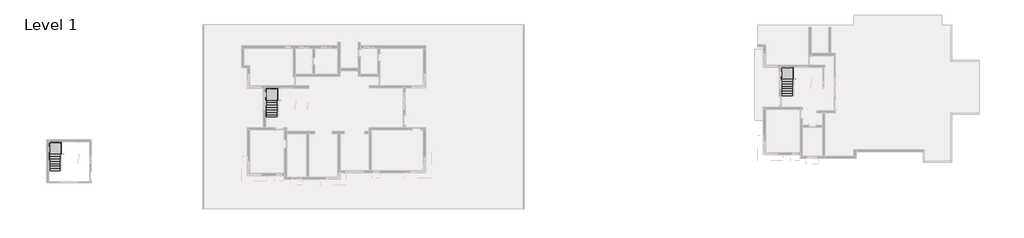
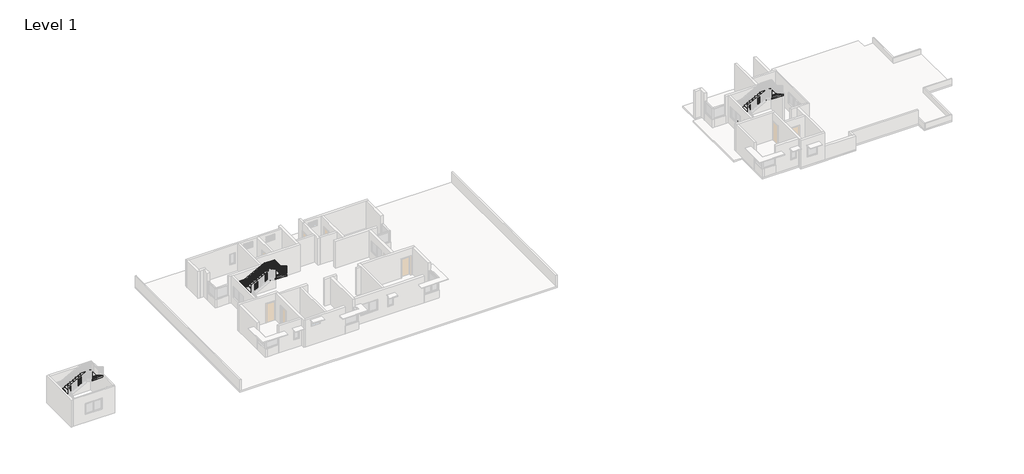
# One storey, part 7 of 9: 3 stair flights, 1 railing.
"""IFC4 building model written with IfcOpenShell, lengths in millimetres."""

from ifc_helpers import new_model, si_unit, frame, origin, place, context, project, spatial, polyline, outline, extrude, faceted_brep, transform, mapped, element, save
from components import stair_flight_18be0a75, stair_flight_c0b809fc, stair_flight_2ad91a83

model = new_model("IFC4")

# Units and contexts
model_context = context("Model", 3, world=origin())
ifc_project = project(units=[si_unit("LENGTHUNIT", "METRE", prefix="MILLI")], contexts=[model_context])

# Site, building, storey
site = spatial("IfcSite", under=ifc_project)
building = spatial("IfcBuilding", under=site)
storey = spatial("IfcBuildingStorey", under=building, Name="Level 1", Elevation=0.0)

# Railing
placement = place(None, origin())
element("IfcRailing", 1, ObjectType="Handrail - Rectangular", at=placement, inside=storey, context=model_context, shape_type="SolidModel", body=[
    faceted_brep([(-40950.9146233, 12415.3624892, 1059.5428571), (-40950.9146233, 12415.3624892, 1001.0339009), (-40900.1146233, 12415.3624892, 1001.0339009), (-40900.1146233, 12415.3624892, 1059.5428571), (-40950.9146233, 14360.1558226, 2170.8533333), (-40950.9146233, 14373.646496, 2120.0533333), (-40900.1146233, 14373.646496, 2120.0533333), (-40900.1146233, 14360.1558226, 2170.8533333), (-40950.9146233, 15412.5624892, 2170.8533333), (-40950.9146233, 15412.5624892, 2120.0533333), (-40900.1146233, 15361.7624892, 2120.0533333), (-40900.1146233, 15361.7624892, 2170.8533333), (-39825.1503376, 15412.5624892, 2170.8533333), (-39812.4503376, 15412.5624892, 2120.0533333), (-39812.4503376, 15361.7624892, 2120.0533333), (-39825.1503376, 15361.7624892, 2170.8533333), (-37733.2789091, 15412.5624892, 3286.5180952), (-37720.5789091, 15412.5624892, 3235.7180952), (-37720.5789091, 15361.7624892, 3235.7180952), (-37733.2789091, 15361.7624892, 3286.5180952), (-36607.5146233, 15412.5624892, 3286.5180952), (-36607.5146233, 15412.5624892, 3235.7180952), (-36658.3146233, 15361.7624892, 3235.7180952), (-36658.3146233, 15361.7624892, 3286.5180952), (-36607.5146233, 14360.1558226, 3286.5180952), (-36607.5146233, 14346.6651492, 3235.7180952), (-36658.3146233, 14346.6651492, 3235.7180952), (-36658.3146233, 14360.1558226, 3286.5180952), (-36607.5146233, 13177.3624892, 3962.4), (-36658.3146233, 13177.3624892, 3962.4), (-36658.3146233, 13177.3624892, 3903.8910438), (-36607.5146233, 13177.3624892, 3903.8910438)], [[[0, 1, 2, 3]], [[1, 0, 4, 5]], [[2, 1, 5, 6]], [[3, 2, 6, 7]], [[0, 3, 7, 4]], [[5, 4, 8, 9]], [[6, 5, 9, 10]], [[7, 6, 10, 11]], [[4, 7, 11, 8]], [[9, 8, 12, 13]], [[10, 9, 13, 14]], [[11, 10, 14, 15]], [[8, 11, 15, 12]], [[13, 12, 16, 17]], [[14, 13, 17, 18]], [[15, 14, 18, 19]], [[12, 15, 19, 16]], [[17, 16, 20, 21]], [[18, 17, 21, 22]], [[19, 18, 22, 23]], [[16, 19, 23, 20]], [[21, 20, 24, 25]], [[22, 21, 25, 26]], [[23, 22, 26, 27]], [[20, 23, 27, 24]], [[28, 29, 30, 31]], [[25, 24, 28, 31]], [[26, 25, 31, 30]], [[27, 26, 30, 29]], [[24, 27, 29, 28]]]),
    extrude(outline(polyline([(13263.0874892, 3854.9053295), (13263.0874892, 2902.8571429), (13244.0374892, 2902.8571429), (13244.0374892, 3865.7910438), (13263.0874892, 3854.9053295)])), frame((-36642.4396233, 0.0, 0.0), z_axis=(1.0, 0.0, 0.0), x_axis=(0.0, 1.0, 0.0)), (0.0, 0.0, 1.0), 19.05),
    extrude(outline(polyline([(13364.6874892, 3796.8481866), (13364.6874892, 2902.8571429), (13345.6374892, 2902.8571429), (13345.6374892, 3807.7339009), (13364.6874892, 3796.8481866)])), frame((-36642.4396233, 0.0, 0.0), z_axis=(1.0, 0.0, 0.0), x_axis=(0.0, 1.0, 0.0)), (0.0, 0.0, 1.0), 19.05),
    extrude(outline(polyline([(13466.2874892, 3738.7910438), (13466.2874892, 2757.7142857), (13447.2374892, 2757.7142857), (13447.2374892, 3749.6767581), (13466.2874892, 3738.7910438)])), frame((-36642.4396233, 0.0, 0.0), z_axis=(1.0, 0.0, 0.0), x_axis=(0.0, 1.0, 0.0)), (0.0, 0.0, 1.0), 19.05),
    extrude(outline(polyline([(13567.8874892, 3680.7339009), (13567.8874892, 2757.7142857), (13548.8374892, 2757.7142857), (13548.8374892, 3691.6196152), (13567.8874892, 3680.7339009)])), frame((-36642.4396233, 0.0, 0.0), z_axis=(1.0, 0.0, 0.0), x_axis=(0.0, 1.0, 0.0)), (0.0, 0.0, 1.0), 19.05),
    extrude(outline(polyline([(13669.4874892, 3622.6767581), (13669.4874892, 2757.7142857), (13650.4374892, 2757.7142857), (13650.4374892, 3633.5624723), (13669.4874892, 3622.6767581)])), frame((-36642.4396233, 0.0, 0.0), z_axis=(1.0, 0.0, 0.0), x_axis=(0.0, 1.0, 0.0)), (0.0, 0.0, 1.0), 19.05),
    extrude(outline(polyline([(13771.0874892, 3564.6196152), (13771.0874892, 2612.5714286), (13752.0374892, 2612.5714286), (13752.0374892, 3575.5053295), (13771.0874892, 3564.6196152)])), frame((-36642.4396233, 0.0, 0.0), z_axis=(1.0, 0.0, 0.0), x_axis=(0.0, 1.0, 0.0)), (0.0, 0.0, 1.0), 19.05),
    extrude(outline(polyline([(13872.6874892, 3506.5624723), (13872.6874892, 2612.5714286), (13853.6374892, 2612.5714286), (13853.6374892, 3517.4481866), (13872.6874892, 3506.5624723)])), frame((-36642.4396233, 0.0, 0.0), z_axis=(1.0, 0.0, 0.0), x_axis=(0.0, 1.0, 0.0)), (0.0, 0.0, 1.0), 19.05),
    extrude(outline(polyline([(13974.2874892, 3448.5053295), (13974.2874892, 2467.4285714), (13955.2374892, 2467.4285714), (13955.2374892, 3459.3910438), (13974.2874892, 3448.5053295)])), frame((-36642.4396233, 0.0, 0.0), z_axis=(1.0, 0.0, 0.0), x_axis=(0.0, 1.0, 0.0)), (0.0, 0.0, 1.0), 19.05),
    extrude(outline(polyline([(14075.8874892, 3390.4481866), (14075.8874892, 2467.4285714), (14056.8374892, 2467.4285714), (14056.8374892, 3401.3339009), (14075.8874892, 3390.4481866)])), frame((-36642.4396233, 0.0, 0.0), z_axis=(1.0, 0.0, 0.0), x_axis=(0.0, 1.0, 0.0)), (0.0, 0.0, 1.0), 19.05),
    extrude(outline(polyline([(14177.4874892, 3332.3910438), (14177.4874892, 2467.4285714), (14158.4374892, 2467.4285714), (14158.4374892, 3343.2767581), (14177.4874892, 3332.3910438)])), frame((-36642.4396233, 0.0, 0.0), z_axis=(1.0, 0.0, 0.0), x_axis=(0.0, 1.0, 0.0)), (0.0, 0.0, 1.0), 19.05),
    extrude(outline(polyline([(14279.0874892, 3274.3339009), (14279.0874892, 2322.2857143), (14260.0374892, 2322.2857143), (14260.0374892, 3285.2196152), (14279.0874892, 3274.3339009)])), frame((-36642.4396233, 0.0, 0.0), z_axis=(1.0, 0.0, 0.0), x_axis=(0.0, 1.0, 0.0)), (0.0, 0.0, 1.0), 19.05),
    extrude(outline(polyline([(-36623.3896233, 14380.6874892), (-36623.3896233, 14361.6374892), (-36642.4396233, 14361.6374892), (-36642.4396233, 14380.6874892), (-36623.3896233, 14380.6874892)])), frame((0.0, 0.0, 2322.2857143), z_axis=(0.0, 0.0, 1.0), x_axis=(1.0, 0.0, 0.0)), (0.0, 0.0, 1.0), 913.432381),
    extrude(outline(polyline([(-36623.3896233, 14482.2874892), (-36623.3896233, 14463.2374892), (-36642.4396233, 14463.2374892), (-36642.4396233, 14482.2874892), (-36623.3896233, 14482.2874892)])), frame((0.0, 0.0, 2322.2857143), z_axis=(0.0, 0.0, 1.0), x_axis=(1.0, 0.0, 0.0)), (0.0, 0.0, 1.0), 913.432381),
    extrude(outline(polyline([(-36623.3896233, 14583.8874892), (-36623.3896233, 14564.8374892), (-36642.4396233, 14564.8374892), (-36642.4396233, 14583.8874892), (-36623.3896233, 14583.8874892)])), frame((0.0, 0.0, 2322.2857143), z_axis=(0.0, 0.0, 1.0), x_axis=(1.0, 0.0, 0.0)), (0.0, 0.0, 1.0), 913.432381),
    extrude(outline(polyline([(-36623.3896233, 14685.4874892), (-36623.3896233, 14666.4374892), (-36642.4396233, 14666.4374892), (-36642.4396233, 14685.4874892), (-36623.3896233, 14685.4874892)])), frame((0.0, 0.0, 2322.2857143), z_axis=(0.0, 0.0, 1.0), x_axis=(1.0, 0.0, 0.0)), (0.0, 0.0, 1.0), 913.432381),
    extrude(outline(polyline([(-36623.3896233, 14787.0874892), (-36623.3896233, 14768.0374892), (-36642.4396233, 14768.0374892), (-36642.4396233, 14787.0874892), (-36623.3896233, 14787.0874892)])), frame((0.0, 0.0, 2322.2857143), z_axis=(0.0, 0.0, 1.0), x_axis=(1.0, 0.0, 0.0)), (0.0, 0.0, 1.0), 913.432381),
    extrude(outline(polyline([(-36623.3896233, 14888.6874892), (-36623.3896233, 14869.6374892), (-36642.4396233, 14869.6374892), (-36642.4396233, 14888.6874892), (-36623.3896233, 14888.6874892)])), frame((0.0, 0.0, 2322.2857143), z_axis=(0.0, 0.0, 1.0), x_axis=(1.0, 0.0, 0.0)), (0.0, 0.0, 1.0), 913.432381),
    extrude(outline(polyline([(-36623.3896233, 14990.2874892), (-36623.3896233, 14971.2374892), (-36642.4396233, 14971.2374892), (-36642.4396233, 14990.2874892), (-36623.3896233, 14990.2874892)])), frame((0.0, 0.0, 2322.2857143), z_axis=(0.0, 0.0, 1.0), x_axis=(1.0, 0.0, 0.0)), (0.0, 0.0, 1.0), 913.432381),
    extrude(outline(polyline([(-36623.3896233, 15091.8874892), (-36623.3896233, 15072.8374892), (-36642.4396233, 15072.8374892), (-36642.4396233, 15091.8874892), (-36623.3896233, 15091.8874892)])), frame((0.0, 0.0, 2322.2857143), z_axis=(0.0, 0.0, 1.0), x_axis=(1.0, 0.0, 0.0)), (0.0, 0.0, 1.0), 913.432381),
    extrude(outline(polyline([(-36623.3896233, 15193.4874892), (-36623.3896233, 15174.4374892), (-36642.4396233, 15174.4374892), (-36642.4396233, 15193.4874892), (-36623.3896233, 15193.4874892)])), frame((0.0, 0.0, 2322.2857143), z_axis=(0.0, 0.0, 1.0), x_axis=(1.0, 0.0, 0.0)), (0.0, 0.0, 1.0), 913.432381),
    extrude(outline(polyline([(-36623.3896233, 15295.0874892), (-36623.3896233, 15276.0374892), (-36642.4396233, 15276.0374892), (-36642.4396233, 15295.0874892), (-36623.3896233, 15295.0874892)])), frame((0.0, 0.0, 2322.2857143), z_axis=(0.0, 0.0, 1.0), x_axis=(1.0, 0.0, 0.0)), (0.0, 0.0, 1.0), 913.432381),
    extrude(outline(polyline([(-36667.8396233, 15396.6874892), (-36648.7896233, 15396.6874892), (-36648.7896233, 15377.6374892), (-36667.8396233, 15377.6374892), (-36667.8396233, 15396.6874892)])), frame((0.0, 0.0, 2322.2857143), z_axis=(0.0, 0.0, 1.0), x_axis=(1.0, 0.0, 0.0)), (0.0, 0.0, 1.0), 913.432381),
    extrude(outline(polyline([(-36769.4396233, 15396.6874892), (-36750.3896233, 15396.6874892), (-36750.3896233, 15377.6374892), (-36769.4396233, 15377.6374892), (-36769.4396233, 15396.6874892)])), frame((0.0, 0.0, 2322.2857143), z_axis=(0.0, 0.0, 1.0), x_axis=(1.0, 0.0, 0.0)), (0.0, 0.0, 1.0), 913.432381),
    extrude(outline(polyline([(-36871.0396233, 15396.6874892), (-36851.9896233, 15396.6874892), (-36851.9896233, 15377.6374892), (-36871.0396233, 15377.6374892), (-36871.0396233, 15396.6874892)])), frame((0.0, 0.0, 2322.2857143), z_axis=(0.0, 0.0, 1.0), x_axis=(1.0, 0.0, 0.0)), (0.0, 0.0, 1.0), 913.432381),
    extrude(outline(polyline([(-36972.6396233, 15396.6874892), (-36953.5896233, 15396.6874892), (-36953.5896233, 15377.6374892), (-36972.6396233, 15377.6374892), (-36972.6396233, 15396.6874892)])), frame((0.0, 0.0, 2322.2857143), z_axis=(0.0, 0.0, 1.0), x_axis=(1.0, 0.0, 0.0)), (0.0, 0.0, 1.0), 913.432381),
    extrude(outline(polyline([(-37074.2396233, 15396.6874892), (-37055.1896233, 15396.6874892), (-37055.1896233, 15377.6374892), (-37074.2396233, 15377.6374892), (-37074.2396233, 15396.6874892)])), frame((0.0, 0.0, 2322.2857143), z_axis=(0.0, 0.0, 1.0), x_axis=(1.0, 0.0, 0.0)), (0.0, 0.0, 1.0), 913.432381),
    extrude(outline(polyline([(-37175.8396233, 15396.6874892), (-37156.7896233, 15396.6874892), (-37156.7896233, 15377.6374892), (-37175.8396233, 15377.6374892), (-37175.8396233, 15396.6874892)])), frame((0.0, 0.0, 2322.2857143), z_axis=(0.0, 0.0, 1.0), x_axis=(1.0, 0.0, 0.0)), (0.0, 0.0, 1.0), 913.432381),
    extrude(outline(polyline([(-37277.4396233, 15396.6874892), (-37258.3896233, 15396.6874892), (-37258.3896233, 15377.6374892), (-37277.4396233, 15377.6374892), (-37277.4396233, 15396.6874892)])), frame((0.0, 0.0, 2322.2857143), z_axis=(0.0, 0.0, 1.0), x_axis=(1.0, 0.0, 0.0)), (0.0, 0.0, 1.0), 913.432381),
    extrude(outline(polyline([(-37379.0396233, 15396.6874892), (-37359.9896233, 15396.6874892), (-37359.9896233, 15377.6374892), (-37379.0396233, 15377.6374892), (-37379.0396233, 15396.6874892)])), frame((0.0, 0.0, 2322.2857143), z_axis=(0.0, 0.0, 1.0), x_axis=(1.0, 0.0, 0.0)), (0.0, 0.0, 1.0), 913.432381),
    extrude(outline(polyline([(-37480.6396233, 15396.6874892), (-37461.5896233, 15396.6874892), (-37461.5896233, 15377.6374892), (-37480.6396233, 15377.6374892), (-37480.6396233, 15396.6874892)])), frame((0.0, 0.0, 2322.2857143), z_axis=(0.0, 0.0, 1.0), x_axis=(1.0, 0.0, 0.0)), (0.0, 0.0, 1.0), 913.432381),
    extrude(outline(polyline([(-37582.2396233, 15396.6874892), (-37563.1896233, 15396.6874892), (-37563.1896233, 15377.6374892), (-37582.2396233, 15377.6374892), (-37582.2396233, 15396.6874892)])), frame((0.0, 0.0, 2322.2857143), z_axis=(0.0, 0.0, 1.0), x_axis=(1.0, 0.0, 0.0)), (0.0, 0.0, 1.0), 913.432381),
    extrude(outline(polyline([(-37683.8396233, 15396.6874892), (-37664.7896233, 15396.6874892), (-37664.7896233, 15377.6374892), (-37683.8396233, 15377.6374892), (-37683.8396233, 15396.6874892)])), frame((0.0, 0.0, 2322.2857143), z_axis=(0.0, 0.0, 1.0), x_axis=(1.0, 0.0, 0.0)), (0.0, 0.0, 1.0), 913.432381),
    extrude(outline(polyline([(3201.1257143, -37785.4396233), (2322.2857143, -37785.4396233), (2322.2857143, -37766.3896233), (3211.2857143, -37766.3896233), (3201.1257143, -37785.4396233)])), frame((0.0, 15377.6374892, 0.0), z_axis=(0.0, 1.0, 0.0), x_axis=(0.0, 0.0, 1.0)), (0.0, 0.0, 1.0), 19.05),
    extrude(outline(polyline([(3146.9390476, -37887.0396233), (2177.1428571, -37887.0396233), (2177.1428571, -37867.9896233), (3157.0990476, -37867.9896233), (3146.9390476, -37887.0396233)])), frame((0.0, 15377.6374892, 0.0), z_axis=(0.0, 1.0, 0.0), x_axis=(0.0, 0.0, 1.0)), (0.0, 0.0, 1.0), 19.05),
    extrude(outline(polyline([(3092.752381, -37988.6396233), (2177.1428571, -37988.6396233), (2177.1428571, -37969.5896233), (3102.912381, -37969.5896233), (3092.752381, -37988.6396233)])), frame((0.0, 15377.6374892, 0.0), z_axis=(0.0, 1.0, 0.0), x_axis=(0.0, 0.0, 1.0)), (0.0, 0.0, 1.0), 19.05),
    extrude(outline(polyline([(3038.5657143, -38090.2396233), (2177.1428571, -38090.2396233), (2177.1428571, -38071.1896233), (3048.7257143, -38071.1896233), (3038.5657143, -38090.2396233)])), frame((0.0, 15377.6374892, 0.0), z_axis=(0.0, 1.0, 0.0), x_axis=(0.0, 0.0, 1.0)), (0.0, 0.0, 1.0), 19.05),
    extrude(outline(polyline([(2984.3790476, -38191.8396233), (2032.0, -38191.8396233), (2032.0, -38172.7896233), (2994.5390476, -38172.7896233), (2984.3790476, -38191.8396233)])), frame((0.0, 15377.6374892, 0.0), z_axis=(0.0, 1.0, 0.0), x_axis=(0.0, 0.0, 1.0)), (0.0, 0.0, 1.0), 19.05),
    extrude(outline(polyline([(2930.192381, -38293.4396233), (2032.0, -38293.4396233), (2032.0, -38274.3896233), (2940.352381, -38274.3896233), (2930.192381, -38293.4396233)])), frame((0.0, 15377.6374892, 0.0), z_axis=(0.0, 1.0, 0.0), x_axis=(0.0, 0.0, 1.0)), (0.0, 0.0, 1.0), 19.05),
    extrude(outline(polyline([(2876.0057143, -38395.0396233), (1886.8571429, -38395.0396233), (1886.8571429, -38375.9896233), (2886.1657143, -38375.9896233), (2876.0057143, -38395.0396233)])), frame((0.0, 15377.6374892, 0.0), z_axis=(0.0, 1.0, 0.0), x_axis=(0.0, 0.0, 1.0)), (0.0, 0.0, 1.0), 19.05),
    extrude(outline(polyline([(2821.8190476, -38496.6396233), (1886.8571429, -38496.6396233), (1886.8571429, -38477.5896233), (2831.9790476, -38477.5896233), (2821.8190476, -38496.6396233)])), frame((0.0, 15377.6374892, 0.0), z_axis=(0.0, 1.0, 0.0), x_axis=(0.0, 0.0, 1.0)), (0.0, 0.0, 1.0), 19.05),
    extrude(outline(polyline([(2767.632381, -38598.2396233), (1886.8571429, -38598.2396233), (1886.8571429, -38579.1896233), (2777.792381, -38579.1896233), (2767.632381, -38598.2396233)])), frame((0.0, 15377.6374892, 0.0), z_axis=(0.0, 1.0, 0.0), x_axis=(0.0, 0.0, 1.0)), (0.0, 0.0, 1.0), 19.05),
    extrude(outline(polyline([(2713.4457143, -38699.8396233), (1741.7142857, -38699.8396233), (1741.7142857, -38680.7896233), (2723.6057143, -38680.7896233), (2713.4457143, -38699.8396233)])), frame((0.0, 15377.6374892, 0.0), z_axis=(0.0, 1.0, 0.0), x_axis=(0.0, 0.0, 1.0)), (0.0, 0.0, 1.0), 19.05),
    extrude(outline(polyline([(2659.2590476, -38801.4396233), (1741.7142857, -38801.4396233), (1741.7142857, -38782.3896233), (2669.4190476, -38782.3896233), (2659.2590476, -38801.4396233)])), frame((0.0, 15377.6374892, 0.0), z_axis=(0.0, 1.0, 0.0), x_axis=(0.0, 0.0, 1.0)), (0.0, 0.0, 1.0), 19.05),
    extrude(outline(polyline([(2605.072381, -38903.0396233), (1741.7142857, -38903.0396233), (1741.7142857, -38883.9896233), (2615.232381, -38883.9896233), (2605.072381, -38903.0396233)])), frame((0.0, 15377.6374892, 0.0), z_axis=(0.0, 1.0, 0.0), x_axis=(0.0, 0.0, 1.0)), (0.0, 0.0, 1.0), 19.05),
    extrude(outline(polyline([(2550.8857143, -39004.6396233), (1596.5714286, -39004.6396233), (1596.5714286, -38985.5896233), (2561.0457143, -38985.5896233), (2550.8857143, -39004.6396233)])), frame((0.0, 15377.6374892, 0.0), z_axis=(0.0, 1.0, 0.0), x_axis=(0.0, 0.0, 1.0)), (0.0, 0.0, 1.0), 19.05),
    extrude(outline(polyline([(2496.6990476, -39106.2396233), (1596.5714286, -39106.2396233), (1596.5714286, -39087.1896233), (2506.8590476, -39087.1896233), (2496.6990476, -39106.2396233)])), frame((0.0, 15377.6374892, 0.0), z_axis=(0.0, 1.0, 0.0), x_axis=(0.0, 0.0, 1.0)), (0.0, 0.0, 1.0), 19.05),
    extrude(outline(polyline([(2442.512381, -39207.8396233), (1596.5714286, -39207.8396233), (1596.5714286, -39188.7896233), (2452.672381, -39188.7896233), (2442.512381, -39207.8396233)])), frame((0.0, 15377.6374892, 0.0), z_axis=(0.0, 1.0, 0.0), x_axis=(0.0, 0.0, 1.0)), (0.0, 0.0, 1.0), 19.05),
    extrude(outline(polyline([(2388.3257143, -39309.4396233), (1451.4285714, -39309.4396233), (1451.4285714, -39290.3896233), (2398.4857143, -39290.3896233), (2388.3257143, -39309.4396233)])), frame((0.0, 15377.6374892, 0.0), z_axis=(0.0, 1.0, 0.0), x_axis=(0.0, 0.0, 1.0)), (0.0, 0.0, 1.0), 19.05),
    extrude(outline(polyline([(2334.1390476, -39411.0396233), (1451.4285714, -39411.0396233), (1451.4285714, -39391.9896233), (2344.2990476, -39391.9896233), (2334.1390476, -39411.0396233)])), frame((0.0, 15377.6374892, 0.0), z_axis=(0.0, 1.0, 0.0), x_axis=(0.0, 0.0, 1.0)), (0.0, 0.0, 1.0), 19.05),
    extrude(outline(polyline([(2279.952381, -39512.6396233), (1306.2857143, -39512.6396233), (1306.2857143, -39493.5896233), (2290.112381, -39493.5896233), (2279.952381, -39512.6396233)])), frame((0.0, 15377.6374892, 0.0), z_axis=(0.0, 1.0, 0.0), x_axis=(0.0, 0.0, 1.0)), (0.0, 0.0, 1.0), 19.05),
    extrude(outline(polyline([(2225.7657143, -39614.2396233), (1306.2857143, -39614.2396233), (1306.2857143, -39595.1896233), (2235.9257143, -39595.1896233), (2225.7657143, -39614.2396233)])), frame((0.0, 15377.6374892, 0.0), z_axis=(0.0, 1.0, 0.0), x_axis=(0.0, 0.0, 1.0)), (0.0, 0.0, 1.0), 19.05),
    extrude(outline(polyline([(2171.5790476, -39715.8396233), (1306.2857143, -39715.8396233), (1306.2857143, -39696.7896233), (2181.7390476, -39696.7896233), (2171.5790476, -39715.8396233)])), frame((0.0, 15377.6374892, 0.0), z_axis=(0.0, 1.0, 0.0), x_axis=(0.0, 0.0, 1.0)), (0.0, 0.0, 1.0), 19.05),
    extrude(outline(polyline([(2117.392381, -39817.4396233), (1161.1428571, -39817.4396233), (1161.1428571, -39798.3896233), (2127.552381, -39798.3896233), (2117.392381, -39817.4396233)])), frame((0.0, 15377.6374892, 0.0), z_axis=(0.0, 1.0, 0.0), x_axis=(0.0, 0.0, 1.0)), (0.0, 0.0, 1.0), 19.05),
    extrude(outline(polyline([(-39919.0396233, 15396.6874892), (-39899.9896233, 15396.6874892), (-39899.9896233, 15377.6374892), (-39919.0396233, 15377.6374892), (-39919.0396233, 15396.6874892)])), frame((0.0, 0.0, 1161.1428571), z_axis=(0.0, 0.0, 1.0), x_axis=(1.0, 0.0, 0.0)), (0.0, 0.0, 1.0), 958.9104762),
    extrude(outline(polyline([(-40020.6396233, 15396.6874892), (-40001.5896233, 15396.6874892), (-40001.5896233, 15377.6374892), (-40020.6396233, 15377.6374892), (-40020.6396233, 15396.6874892)])), frame((0.0, 0.0, 1161.1428571), z_axis=(0.0, 0.0, 1.0), x_axis=(1.0, 0.0, 0.0)), (0.0, 0.0, 1.0), 958.9104762),
    extrude(outline(polyline([(-40122.2396233, 15396.6874892), (-40103.1896233, 15396.6874892), (-40103.1896233, 15377.6374892), (-40122.2396233, 15377.6374892), (-40122.2396233, 15396.6874892)])), frame((0.0, 0.0, 1161.1428571), z_axis=(0.0, 0.0, 1.0), x_axis=(1.0, 0.0, 0.0)), (0.0, 0.0, 1.0), 958.9104762),
    extrude(outline(polyline([(-40223.8396233, 15396.6874892), (-40204.7896233, 15396.6874892), (-40204.7896233, 15377.6374892), (-40223.8396233, 15377.6374892), (-40223.8396233, 15396.6874892)])), frame((0.0, 0.0, 1161.1428571), z_axis=(0.0, 0.0, 1.0), x_axis=(1.0, 0.0, 0.0)), (0.0, 0.0, 1.0), 958.9104762),
    extrude(outline(polyline([(-40325.4396233, 15396.6874892), (-40306.3896233, 15396.6874892), (-40306.3896233, 15377.6374892), (-40325.4396233, 15377.6374892), (-40325.4396233, 15396.6874892)])), frame((0.0, 0.0, 1161.1428571), z_axis=(0.0, 0.0, 1.0), x_axis=(1.0, 0.0, 0.0)), (0.0, 0.0, 1.0), 958.9104762),
    extrude(outline(polyline([(-40427.0396233, 15396.6874892), (-40407.9896233, 15396.6874892), (-40407.9896233, 15377.6374892), (-40427.0396233, 15377.6374892), (-40427.0396233, 15396.6874892)])), frame((0.0, 0.0, 1161.1428571), z_axis=(0.0, 0.0, 1.0), x_axis=(1.0, 0.0, 0.0)), (0.0, 0.0, 1.0), 958.9104762),
    extrude(outline(polyline([(-40528.6396233, 15396.6874892), (-40509.5896233, 15396.6874892), (-40509.5896233, 15377.6374892), (-40528.6396233, 15377.6374892), (-40528.6396233, 15396.6874892)])), frame((0.0, 0.0, 1161.1428571), z_axis=(0.0, 0.0, 1.0), x_axis=(1.0, 0.0, 0.0)), (0.0, 0.0, 1.0), 958.9104762),
    extrude(outline(polyline([(-40630.2396233, 15396.6874892), (-40611.1896233, 15396.6874892), (-40611.1896233, 15377.6374892), (-40630.2396233, 15377.6374892), (-40630.2396233, 15396.6874892)])), frame((0.0, 0.0, 1161.1428571), z_axis=(0.0, 0.0, 1.0), x_axis=(1.0, 0.0, 0.0)), (0.0, 0.0, 1.0), 958.9104762),
    extrude(outline(polyline([(-40731.8396233, 15396.6874892), (-40712.7896233, 15396.6874892), (-40712.7896233, 15377.6374892), (-40731.8396233, 15377.6374892), (-40731.8396233, 15396.6874892)])), frame((0.0, 0.0, 1161.1428571), z_axis=(0.0, 0.0, 1.0), x_axis=(1.0, 0.0, 0.0)), (0.0, 0.0, 1.0), 958.9104762),
    extrude(outline(polyline([(-40833.4396233, 15396.6874892), (-40814.3896233, 15396.6874892), (-40814.3896233, 15377.6374892), (-40833.4396233, 15377.6374892), (-40833.4396233, 15396.6874892)])), frame((0.0, 0.0, 1161.1428571), z_axis=(0.0, 0.0, 1.0), x_axis=(1.0, 0.0, 0.0)), (0.0, 0.0, 1.0), 958.9104762),
    extrude(outline(polyline([(-40935.0396233, 15352.2374892), (-40935.0396233, 15371.2874892), (-40915.9896233, 15371.2874892), (-40915.9896233, 15352.2374892), (-40935.0396233, 15352.2374892)])), frame((0.0, 0.0, 1161.1428571), z_axis=(0.0, 0.0, 1.0), x_axis=(1.0, 0.0, 0.0)), (0.0, 0.0, 1.0), 958.9104762),
    extrude(outline(polyline([(-40935.0396233, 15250.6374892), (-40935.0396233, 15269.6874892), (-40915.9896233, 15269.6874892), (-40915.9896233, 15250.6374892), (-40935.0396233, 15250.6374892)])), frame((0.0, 0.0, 1161.1428571), z_axis=(0.0, 0.0, 1.0), x_axis=(1.0, 0.0, 0.0)), (0.0, 0.0, 1.0), 958.9104762),
    extrude(outline(polyline([(-40935.0396233, 15149.0374892), (-40935.0396233, 15168.0874892), (-40915.9896233, 15168.0874892), (-40915.9896233, 15149.0374892), (-40935.0396233, 15149.0374892)])), frame((0.0, 0.0, 1161.1428571), z_axis=(0.0, 0.0, 1.0), x_axis=(1.0, 0.0, 0.0)), (0.0, 0.0, 1.0), 958.9104762),
    extrude(outline(polyline([(-40935.0396233, 15047.4374892), (-40935.0396233, 15066.4874892), (-40915.9896233, 15066.4874892), (-40915.9896233, 15047.4374892), (-40935.0396233, 15047.4374892)])), frame((0.0, 0.0, 1161.1428571), z_axis=(0.0, 0.0, 1.0), x_axis=(1.0, 0.0, 0.0)), (0.0, 0.0, 1.0), 958.9104762),
    extrude(outline(polyline([(-40935.0396233, 14945.8374892), (-40935.0396233, 14964.8874892), (-40915.9896233, 14964.8874892), (-40915.9896233, 14945.8374892), (-40935.0396233, 14945.8374892)])), frame((0.0, 0.0, 1161.1428571), z_axis=(0.0, 0.0, 1.0), x_axis=(1.0, 0.0, 0.0)), (0.0, 0.0, 1.0), 958.9104762),
    extrude(outline(polyline([(-40935.0396233, 14844.2374892), (-40935.0396233, 14863.2874892), (-40915.9896233, 14863.2874892), (-40915.9896233, 14844.2374892), (-40935.0396233, 14844.2374892)])), frame((0.0, 0.0, 1161.1428571), z_axis=(0.0, 0.0, 1.0), x_axis=(1.0, 0.0, 0.0)), (0.0, 0.0, 1.0), 958.9104762),
    extrude(outline(polyline([(-40935.0396233, 14742.6374892), (-40935.0396233, 14761.6874892), (-40915.9896233, 14761.6874892), (-40915.9896233, 14742.6374892), (-40935.0396233, 14742.6374892)])), frame((0.0, 0.0, 1161.1428571), z_axis=(0.0, 0.0, 1.0), x_axis=(1.0, 0.0, 0.0)), (0.0, 0.0, 1.0), 958.9104762),
    extrude(outline(polyline([(-40935.0396233, 14641.0374892), (-40935.0396233, 14660.0874892), (-40915.9896233, 14660.0874892), (-40915.9896233, 14641.0374892), (-40935.0396233, 14641.0374892)])), frame((0.0, 0.0, 1161.1428571), z_axis=(0.0, 0.0, 1.0), x_axis=(1.0, 0.0, 0.0)), (0.0, 0.0, 1.0), 958.9104762),
    extrude(outline(polyline([(-40935.0396233, 14539.4374892), (-40935.0396233, 14558.4874892), (-40915.9896233, 14558.4874892), (-40915.9896233, 14539.4374892), (-40935.0396233, 14539.4374892)])), frame((0.0, 0.0, 1161.1428571), z_axis=(0.0, 0.0, 1.0), x_axis=(1.0, 0.0, 0.0)), (0.0, 0.0, 1.0), 958.9104762),
    extrude(outline(polyline([(-40935.0396233, 14437.8374892), (-40935.0396233, 14456.8874892), (-40915.9896233, 14456.8874892), (-40915.9896233, 14437.8374892), (-40935.0396233, 14437.8374892)])), frame((0.0, 0.0, 1161.1428571), z_axis=(0.0, 0.0, 1.0), x_axis=(1.0, 0.0, 0.0)), (0.0, 0.0, 1.0), 958.9104762),
    extrude(outline(polyline([(14355.2874892, 2109.5624723), (14355.2874892, 1161.1428571), (14336.2374892, 1161.1428571), (14336.2374892, 2098.6767581), (14355.2874892, 2109.5624723)])), frame((-40935.0396233, 0.0, 0.0), z_axis=(1.0, 0.0, 0.0), x_axis=(0.0, 1.0, 0.0)), (0.0, 0.0, 1.0), 19.05),
    extrude(outline(polyline([(14253.6874892, 2051.5053295), (14253.6874892, 1161.1428571), (14234.6374892, 1161.1428571), (14234.6374892, 2040.6196152), (14253.6874892, 2051.5053295)])), frame((-40935.0396233, 0.0, 0.0), z_axis=(1.0, 0.0, 0.0), x_axis=(0.0, 1.0, 0.0)), (0.0, 0.0, 1.0), 19.05),
    extrude(outline(polyline([(14152.0874892, 1993.4481866), (14152.0874892, 1016.0), (14133.0374892, 1016.0), (14133.0374892, 1982.5624723), (14152.0874892, 1993.4481866)])), frame((-40935.0396233, 0.0, 0.0), z_axis=(1.0, 0.0, 0.0), x_axis=(0.0, 1.0, 0.0)), (0.0, 0.0, 1.0), 19.05),
    extrude(outline(polyline([(14050.4874892, 1935.3910438), (14050.4874892, 1016.0), (14031.4374892, 1016.0), (14031.4374892, 1924.5053295), (14050.4874892, 1935.3910438)])), frame((-40935.0396233, 0.0, 0.0), z_axis=(1.0, 0.0, 0.0), x_axis=(0.0, 1.0, 0.0)), (0.0, 0.0, 1.0), 19.05),
    extrude(outline(polyline([(13948.8874892, 1877.3339009), (13948.8874892, 1016.0), (13929.8374892, 1016.0), (13929.8374892, 1866.4481866), (13948.8874892, 1877.3339009)])), frame((-40935.0396233, 0.0, 0.0), z_axis=(1.0, 0.0, 0.0), x_axis=(0.0, 1.0, 0.0)), (0.0, 0.0, 1.0), 19.05),
    extrude(outline(polyline([(13847.2874892, 1819.2767581), (13847.2874892, 870.8571429), (13828.2374892, 870.8571429), (13828.2374892, 1808.3910438), (13847.2874892, 1819.2767581)])), frame((-40935.0396233, 0.0, 0.0), z_axis=(1.0, 0.0, 0.0), x_axis=(0.0, 1.0, 0.0)), (0.0, 0.0, 1.0), 19.05),
    extrude(outline(polyline([(13745.6874892, 1761.2196152), (13745.6874892, 870.8571429), (13726.6374892, 870.8571429), (13726.6374892, 1750.3339009), (13745.6874892, 1761.2196152)])), frame((-40935.0396233, 0.0, 0.0), z_axis=(1.0, 0.0, 0.0), x_axis=(0.0, 1.0, 0.0)), (0.0, 0.0, 1.0), 19.05),
    extrude(outline(polyline([(13644.0874892, 1703.1624723), (13644.0874892, 725.7142857), (13625.0374892, 725.7142857), (13625.0374892, 1692.2767581), (13644.0874892, 1703.1624723)])), frame((-40935.0396233, 0.0, 0.0), z_axis=(1.0, 0.0, 0.0), x_axis=(0.0, 1.0, 0.0)), (0.0, 0.0, 1.0), 19.05),
    extrude(outline(polyline([(13542.4874892, 1645.1053295), (13542.4874892, 725.7142857), (13523.4374892, 725.7142857), (13523.4374892, 1634.2196152), (13542.4874892, 1645.1053295)])), frame((-40935.0396233, 0.0, 0.0), z_axis=(1.0, 0.0, 0.0), x_axis=(0.0, 1.0, 0.0)), (0.0, 0.0, 1.0), 19.05),
    extrude(outline(polyline([(13440.8874892, 1587.0481866), (13440.8874892, 725.7142857), (13421.8374892, 725.7142857), (13421.8374892, 1576.1624723), (13440.8874892, 1587.0481866)])), frame((-40935.0396233, 0.0, 0.0), z_axis=(1.0, 0.0, 0.0), x_axis=(0.0, 1.0, 0.0)), (0.0, 0.0, 1.0), 19.05),
    extrude(outline(polyline([(13339.2874892, 1528.9910438), (13339.2874892, 580.5714286), (13320.2374892, 580.5714286), (13320.2374892, 1518.1053295), (13339.2874892, 1528.9910438)])), frame((-40935.0396233, 0.0, 0.0), z_axis=(1.0, 0.0, 0.0), x_axis=(0.0, 1.0, 0.0)), (0.0, 0.0, 1.0), 19.05),
    extrude(outline(polyline([(13237.6874892, 1470.9339009), (13237.6874892, 580.5714286), (13218.6374892, 580.5714286), (13218.6374892, 1460.0481866), (13237.6874892, 1470.9339009)])), frame((-40935.0396233, 0.0, 0.0), z_axis=(1.0, 0.0, 0.0), x_axis=(0.0, 1.0, 0.0)), (0.0, 0.0, 1.0), 19.05),
    extrude(outline(polyline([(13136.0874892, 1412.8767581), (13136.0874892, 435.4285714), (13117.0374892, 435.4285714), (13117.0374892, 1401.9910438), (13136.0874892, 1412.8767581)])), frame((-40935.0396233, 0.0, 0.0), z_axis=(1.0, 0.0, 0.0), x_axis=(0.0, 1.0, 0.0)), (0.0, 0.0, 1.0), 19.05),
    extrude(outline(polyline([(13034.4874892, 1354.8196152), (13034.4874892, 435.4285714), (13015.4374892, 435.4285714), (13015.4374892, 1343.9339009), (13034.4874892, 1354.8196152)])), frame((-40935.0396233, 0.0, 0.0), z_axis=(1.0, 0.0, 0.0), x_axis=(0.0, 1.0, 0.0)), (0.0, 0.0, 1.0), 19.05),
    extrude(outline(polyline([(12932.8874892, 1296.7624723), (12932.8874892, 435.4285714), (12913.8374892, 435.4285714), (12913.8374892, 1285.8767581), (12932.8874892, 1296.7624723)])), frame((-40935.0396233, 0.0, 0.0), z_axis=(1.0, 0.0, 0.0), x_axis=(0.0, 1.0, 0.0)), (0.0, 0.0, 1.0), 19.05),
    extrude(outline(polyline([(12831.2874892, 1238.7053295), (12831.2874892, 290.2857143), (12812.2374892, 290.2857143), (12812.2374892, 1227.8196152), (12831.2874892, 1238.7053295)])), frame((-40935.0396233, 0.0, 0.0), z_axis=(1.0, 0.0, 0.0), x_axis=(0.0, 1.0, 0.0)), (0.0, 0.0, 1.0), 19.05),
    extrude(outline(polyline([(12729.6874892, 1180.6481866), (12729.6874892, 290.2857143), (12710.6374892, 290.2857143), (12710.6374892, 1169.7624723), (12729.6874892, 1180.6481866)])), frame((-40935.0396233, 0.0, 0.0), z_axis=(1.0, 0.0, 0.0), x_axis=(0.0, 1.0, 0.0)), (0.0, 0.0, 1.0), 19.05),
    extrude(outline(polyline([(12628.0874892, 1122.5910438), (12628.0874892, 145.1428571), (12609.0374892, 145.1428571), (12609.0374892, 1111.7053295), (12628.0874892, 1122.5910438)])), frame((-40935.0396233, 0.0, 0.0), z_axis=(1.0, 0.0, 0.0), x_axis=(0.0, 1.0, 0.0)), (0.0, 0.0, 1.0), 19.05),
    extrude(outline(polyline([(12526.4874892, 1064.5339009), (12526.4874892, 145.1428571), (12507.4374892, 145.1428571), (12507.4374892, 1053.6481866), (12526.4874892, 1064.5339009)])), frame((-40935.0396233, 0.0, 0.0), z_axis=(1.0, 0.0, 0.0), x_axis=(0.0, 1.0, 0.0)), (0.0, 0.0, 1.0), 19.05),
    extrude(outline(polyline([(-36642.4396233, 15396.6874892), (-36623.3896233, 15396.6874892), (-36623.3896233, 15377.6374892), (-36642.4396233, 15377.6374892), (-36642.4396233, 15396.6874892)])), frame((0.0, 0.0, 2322.2857143), z_axis=(0.0, 0.0, 1.0), x_axis=(1.0, 0.0, 0.0)), (0.0, 0.0, 1.0), 913.432381),
    extrude(outline(polyline([(-40935.0396233, 15377.6374892), (-40935.0396233, 15396.6874892), (-40915.9896233, 15396.6874892), (-40915.9896233, 15377.6374892), (-40935.0396233, 15377.6374892)])), frame((0.0, 0.0, 1161.1428571), z_axis=(0.0, 0.0, 1.0), x_axis=(1.0, 0.0, 0.0)), (0.0, 0.0, 1.0), 958.9104762),
    extrude(outline(polyline([(13196.4124892, 3893.0053295), (13196.4124892, 2902.8571429), (13177.3624892, 2902.8571429), (13177.3624892, 3903.8910438), (13196.4124892, 3893.0053295)])), frame((-36642.4396233, 0.0, 0.0), z_axis=(1.0, 0.0, 0.0), x_axis=(0.0, 1.0, 0.0)), (0.0, 0.0, 1.0), 19.05),
    extrude(outline(polyline([(12434.4124892, 1011.9196152), (12434.4124892, 145.1428571), (12415.3624892, 145.1428571), (12415.3624892, 1001.0339009), (12434.4124892, 1011.9196152)])), frame((-40935.0396233, 0.0, 0.0), z_axis=(1.0, 0.0, 0.0), x_axis=(0.0, 1.0, 0.0)), (0.0, 0.0, 1.0), 19.05),
])

# Stair flights
stair_flight_shape = stair_flight_18be0a75(model_context)
element("IfcStairFlight", 2, ObjectType="2\" Tread 1\" Nosing 1/4\" Riser", at=placement, inside=storey, context=model_context, shape_type="MappedRepresentation", body=[
    mapped(stair_flight_shape, transform((0.0, 0.0, 0.0), x_axis=(1.0, 0.0, 0.0), y_axis=(0.0, 1.0, 0.0), z_axis=(0.0, 0.0, 1.0))),
])
stair_flight_2_shape = stair_flight_c0b809fc(model_context)
element("IfcStairFlight", 3, ObjectType="2\" Tread 1\" Nosing 1/4\" Riser", at=placement, inside=storey, context=model_context, shape_type="MappedRepresentation", body=[
    mapped(stair_flight_2_shape, transform((0.0, 0.0, 0.0), x_axis=(1.0, 0.0, 0.0), y_axis=(0.0, 1.0, 0.0), z_axis=(0.0, 0.0, 1.0))),
])
stair_flight_3_shape = stair_flight_2ad91a83(model_context)
element("IfcStairFlight", 4, ObjectType="2\" Tread 1\" Nosing 1/4\" Riser", at=placement, inside=storey, context=model_context, shape_type="MappedRepresentation", body=[
    mapped(stair_flight_3_shape, transform((0.0, 0.0, 0.0), x_axis=(1.0, 0.0, 0.0), y_axis=(0.0, 1.0, 0.0), z_axis=(0.0, 0.0, 1.0))),
])

save(model, "model.ifc")

# Revit data of these elements
# Type "Handrail - Rectangular"
#   Assembly Code = "C2010400"
#   built-in parameter 1008612 = 0.0416667 (stored number, unit not read)
#   built-in parameter 1008611 = 0.0416667 (stored number, unit not read)
#   built-in parameter 1008609 = 0.333333 (stored number, unit not read)
#   built-in parameter 1008604 = 0.166667 (stored number, unit not read)
#   built-in parameter 1008603 = 0.166667 (stored number, unit not read)
#   Railing Height = 3' - 0"
#   built-in parameter 1008630 = 2
#   built-in parameter 1008610 = 2
#   built-in parameter 1008618 = Baluster - Square : 3/4"
# Element 1 (IfcRailing, "Handrail - Rectangular")
#   Phase Created = New Construction
# Elements 2, 3, 4 (IfcStairFlight, "2\" Tread 1\" Nosing 1/4\" Riser")
#   Phase Created = New Construction
